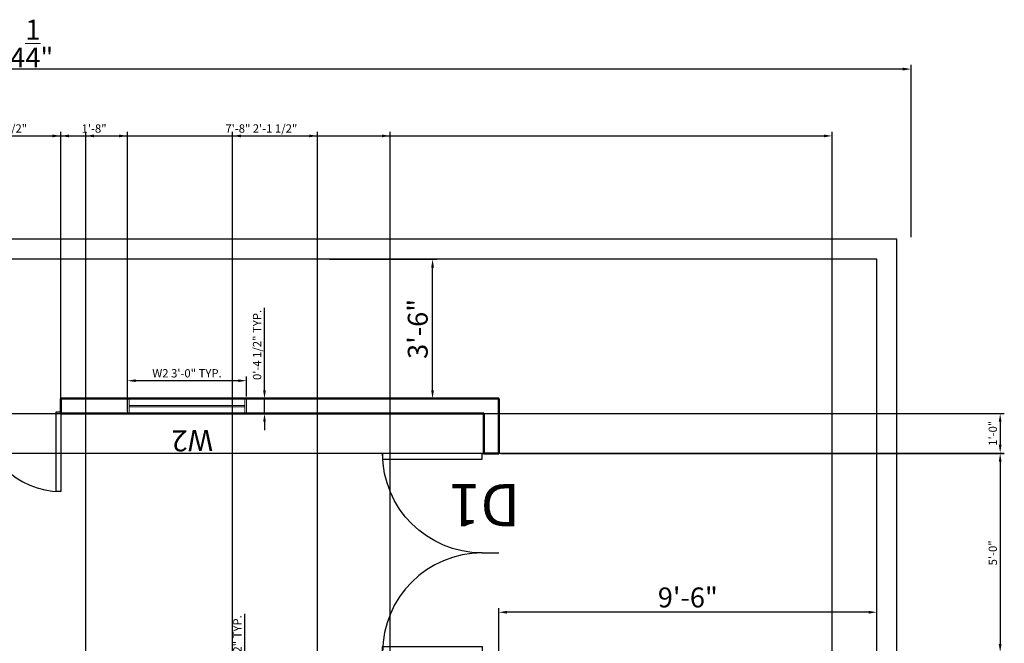
# Model space of a CAD drawing. Units: inches. Extents: x 1989 to 2637, y 1032 to 1611.
# Tile 5 of 5: x 2340 to 2637, y 1423 to 1611. Entities that reach past the tile are written whole.
import ezdxf

# ---------------------------------------------------------------- set-up
doc = ezdxf.new("R2010")
doc.units = ezdxf.units.IN
for name, color, linetype, lineweight in [('A-ANNO-TEXT', 1, 'Continuous', 18), ('C-PROP', 7, 'Continuous', 25), ('DIMENSIONS', 7, 'Continuous', 18), ('doors', 5, 'Continuous', 25), ('walls', 7, 'Continuous', 50), ('windows', 3, 'Continuous', 18)]:
    doc.layers.add(name, color=color, linetype=linetype, lineweight=lineweight)
doc.styles.get("Standard").update_dxf_attribs({"font": 'arial.ttf'})
doc.dimstyles.new('ISO-25', dxfattribs={"dimtxt": 2.5, "dimasz": 2.5, "dimexe": 1.25, "dimexo": 0.625, "dimtad": 1, "dimlunit": 4, "dimtxsty": 'Standard', "dimcen": 2.5, "dimadec": 0, "dimazin": 0, "dimtfac": 1, "dimtmove": 0, "dimatfit": 3, "dimfxl": 1, "dimarcsym": 0})

# ---------------------------------------------------------------- blocks, each defined once
blk = doc.blocks.new('*U2')
for p, q in [((0, 0), (0, -5)), ((30, 0), (30, -5))]:
    blk.add_line(p, q)
blk.add_lwpolyline([(0, 0), (0, 30), (1.75, 30), (1.75, 0)], close=True)
blk.add_arc((0, 0), 30, 0, 90)
blk = doc.blocks.new('*D12')
at = {"layer": 'Defpoints', "color": 0, "transparency": 16777216}
for p in [(2064.5, 1596.21), (2064.5, 1544.92), (2608.81, 1544.92)]:
    blk.add_point(p, dxfattribs=at)
at = {"layer": 'DIMENSIONS', "color": 0, "lineweight": -2, "transparency": 16777216}
for p, q in [((2064.5, 1545.55), (2064.5, 1597.46)), ((2608.81, 1545.55), (2608.81, 1597.46)), ((2606.31, 1596.21), (2067, 1596.21))]:
    blk.add_line(p, q, dxfattribs=at)
at = {"layer": 'DIMENSIONS', "color": 0, "transparency": 16777216}
for points in [[(2067, 1596.63), (2067, 1595.79), (2064.5, 1596.21)], [(2606.31, 1596.63), (2606.31, 1595.79), (2608.81, 1596.21)]]:
    blk.add_solid(points, dxfattribs=at)
at = {"layer": 'DIMENSIONS', "color": 0, "transparency": 16777216, "insert": (2336.65, 1603.9), "char_height": 6, "attachment_point": 5}
blk.add_mtext('45\'-4{\\H1x;\\S1/4;}"', dxfattribs=at)
blk = doc.blocks.new('*D13')
at = {"layer": 'Defpoints', "color": 0, "transparency": 16777216}
for p in [(2484.5, 1432.53), (2484.5, 1402.72), (2598.5, 1403.71)]:
    blk.add_point(p, dxfattribs=at)
at = {"layer": 'DIMENSIONS', "color": 0, "lineweight": -2, "transparency": 16777216}
for p, q in [((2484.5, 1403.34), (2484.5, 1433.78)), ((2598.5, 1404.33), (2598.5, 1433.78)), ((2596, 1432.53), (2487, 1432.53))]:
    blk.add_line(p, q, dxfattribs=at)
at = {"layer": 'DIMENSIONS', "color": 0, "transparency": 16777216}
for points in [[(2487, 1432.95), (2487, 1432.12), (2484.5, 1432.53)], [(2596, 1432.95), (2596, 1432.12), (2598.5, 1432.53)]]:
    blk.add_solid(points, dxfattribs=at)
at = {"layer": 'DIMENSIONS', "color": 0, "transparency": 16777216, "insert": (2541.5, 1436.22), "char_height": 6, "attachment_point": 5}
blk.add_mtext('9\'-6"', dxfattribs=at)
blk = doc.blocks.new('*D14')
at = {"layer": 'Defpoints', "color": 0, "transparency": 16777216}
for p in [(2432.92, 1538.92), (2464.56, 1538.92), (2432.92, 1496.92)]:
    blk.add_point(p, dxfattribs=at)
at = {"layer": 'DIMENSIONS', "color": 0, "lineweight": -2, "transparency": 16777216}
for p, q in [((2433.54, 1538.92), (2465.81, 1538.92)), ((2464.56, 1499.42), (2464.56, 1536.42)), ((2433.54, 1496.92), (2465.81, 1496.92))]:
    blk.add_line(p, q, dxfattribs=at)
at = {"layer": 'DIMENSIONS', "color": 0, "transparency": 16777216}
for points in [[(2464.14, 1536.42), (2464.98, 1536.42), (2464.56, 1538.92)], [(2464.14, 1499.42), (2464.98, 1499.42), (2464.56, 1496.92)]]:
    blk.add_solid(points, dxfattribs=at)
at = {"layer": 'DIMENSIONS', "color": 0, "transparency": 16777216, "insert": (2460.87, 1517.92), "char_height": 6, "attachment_point": 5, "rotation": 90}
blk.add_mtext('3\'-6"', dxfattribs=at)
blk = doc.blocks.new('WIN-W2-36IN')
for p, q in [((0, 0), (0, 35.95)), ((0, 35.95), (4.5, 35.95)), ((4.5, 35.95), (4.5, 0)), ((0, 35.45), (4.5, 35.45)), ((2.05, 35.45), (2.05, 0.5)), ((2.45, 35.45), (2.45, 0.5)), ((4.5, 0.5), (0, 0.5)), ((4.5, 0), (0, 0))]:
    blk.add_line(p, q)
blk = doc.blocks.new('*D26')
at = {"layer": 'Defpoints', "color": 0, "transparency": 16777216}
for p in [(2372.56, 1502.31), (2372.56, 1496.92), (2408.51, 1496.92)]:
    blk.add_point(p, dxfattribs=at)
at = {"layer": 'DIMENSIONS', "color": 0, "lineweight": -2, "transparency": 16777216}
for p, q in [((2372.56, 1497.55), (2372.56, 1503.56)), ((2406.01, 1502.31), (2375.06, 1502.31)), ((2408.51, 1497.55), (2408.51, 1503.56))]:
    blk.add_line(p, q, dxfattribs=at)
at = {"layer": 'DIMENSIONS', "color": 0, "transparency": 16777216}
for points in [[(2375.06, 1502.73), (2375.06, 1501.9), (2372.56, 1502.31)], [(2406.01, 1502.73), (2406.01, 1501.9), (2408.51, 1502.31)]]:
    blk.add_solid(points, dxfattribs=at)
at = {"layer": 'DIMENSIONS', "color": 0, "transparency": 16777216, "insert": (2390.54, 1504.22), "char_height": 2.5, "attachment_point": 5}
blk.add_mtext('W2 3\'-0" TYP.', dxfattribs=at)
blk = doc.blocks.new('*D27')
at = {"layer": 'Defpoints', "color": 0, "transparency": 16777216}
for p in [(2408.51, 1496.92), (2413.9, 1496.92), (2408.51, 1492.42)]:
    blk.add_point(p, dxfattribs=at)
at = {"layer": 'DIMENSIONS', "color": 0, "lineweight": -2, "transparency": 16777216}
for p, q in [((2413.9, 1499.42), (2413.9, 1524.23)), ((2409.14, 1496.92), (2415.15, 1496.92)), ((2413.9, 1492.42), (2413.9, 1496.92)), ((2409.14, 1492.42), (2415.15, 1492.42)), ((2413.9, 1489.92), (2413.9, 1487.42))]:
    blk.add_line(p, q, dxfattribs=at)
at = {"layer": 'DIMENSIONS', "color": 0, "transparency": 16777216}
for points in [[(2413.49, 1499.42), (2414.32, 1499.42), (2413.9, 1496.92)], [(2413.49, 1489.92), (2414.32, 1489.92), (2413.9, 1492.42)]]:
    blk.add_solid(points, dxfattribs=at)
at = {"layer": 'DIMENSIONS', "color": 0, "transparency": 16777216, "insert": (2411.99, 1513.08), "char_height": 2.5, "attachment_point": 5, "rotation": 90}
blk.add_mtext('0\'-4 1/2" TYP.', dxfattribs=at)
blk = doc.blocks.new('*D29')
at = {"layer": 'Defpoints', "color": 0, "transparency": 16777216}
for p in [(2407.97, 1407.51), (2411.12, 1407.51), (2411.12, 1390.17)]:
    blk.add_point(p, dxfattribs=at)
at = {"layer": 'DIMENSIONS', "color": 0, "lineweight": -2, "transparency": 16777216}
for p, q in [((2407.97, 1407.51), (2407.97, 1432.09)), ((2410.49, 1407.51), (2406.72, 1407.51)), ((2407.97, 1392.67), (2407.97, 1405.01)), ((2410.49, 1390.17), (2406.72, 1390.17))]:
    blk.add_line(p, q, dxfattribs=at)
at = {"layer": 'DIMENSIONS', "color": 0, "transparency": 16777216}
for points in [[(2407.55, 1405.01), (2408.39, 1405.01), (2407.97, 1407.51)], [(2407.55, 1392.67), (2408.39, 1392.67), (2407.97, 1390.17)]]:
    blk.add_solid(points, dxfattribs=at)
at = {"layer": 'DIMENSIONS', "color": 0, "transparency": 16777216, "insert": (2406.05, 1421.05), "char_height": 2.5, "attachment_point": 5, "rotation": 90}
blk.add_mtext('1\'-5 1/2" TYP.', dxfattribs=at)
blk = doc.blocks.new('*D40')
at = {"layer": 'Defpoints', "color": 0, "transparency": 16777216}
for p in [(2585, 1576.07), (2082.5, 1496.92), (2585, 1310.92)]:
    blk.add_point(p, dxfattribs=at)
at = {"layer": 'DIMENSIONS', "color": 0, "lineweight": -2, "transparency": 16777216}
for p, q in [((2082.5, 1497.55), (2082.5, 1577.32)), ((2085, 1576.07), (2582.5, 1576.07)), ((2585, 1311.55), (2585, 1577.32))]:
    blk.add_line(p, q, dxfattribs=at)
at = {"layer": 'DIMENSIONS', "color": 0, "transparency": 16777216}
for points in [[(2085, 1576.49), (2085, 1575.65), (2082.5, 1576.07)], [(2582.5, 1576.49), (2582.5, 1575.65), (2585, 1576.07)]]:
    blk.add_solid(points, dxfattribs=at)
at = {"layer": 'DIMENSIONS', "color": 0, "transparency": 16777216, "insert": (2333.75, 1577.99), "char_height": 2.5, "attachment_point": 5}
blk.add_mtext('41\'-10 1/2"', dxfattribs=at)
blk = doc.blocks.new('*D42')
at = {"layer": 'Defpoints', "color": 0, "transparency": 16777216}
for p in [(2484.5, 1480.42), (2484.5, 1420.42), (2635.65, 1420.42)]:
    blk.add_point(p, dxfattribs=at)
at = {"layer": 'DIMENSIONS', "color": 0, "lineweight": -2, "transparency": 16777216}
for p, q in [((2485.12, 1480.42), (2636.9, 1480.42)), ((2635.65, 1477.92), (2635.65, 1422.92)), ((2485.12, 1420.42), (2636.9, 1420.42))]:
    blk.add_line(p, q, dxfattribs=at)
at = {"layer": 'DIMENSIONS', "color": 0, "transparency": 16777216}
for points in [[(2635.23, 1477.92), (2636.06, 1477.92), (2635.65, 1480.42)], [(2635.23, 1422.92), (2636.06, 1422.92), (2635.65, 1420.42)]]:
    blk.add_solid(points, dxfattribs=at)
at = {"layer": 'DIMENSIONS', "color": 0, "transparency": 16777216, "insert": (2633.75, 1450.42), "char_height": 2.5, "attachment_point": 5, "rotation": 90}
blk.add_mtext('5\'-0"', dxfattribs=at)
blk = doc.blocks.new('*D44')
at = {"layer": 'Defpoints', "color": 0, "transparency": 16777216}
for p in [(2352.5, 1576.07), (2304.5, 1496.92), (2352.5, 1496.92)]:
    blk.add_point(p, dxfattribs=at)
at = {"layer": 'DIMENSIONS', "color": 0, "lineweight": -2, "transparency": 16777216}
for p, q in [((2304.5, 1497.55), (2304.5, 1577.32)), ((2307, 1576.07), (2350, 1576.07)), ((2352.5, 1497.55), (2352.5, 1577.32))]:
    blk.add_line(p, q, dxfattribs=at)
at = {"layer": 'DIMENSIONS', "color": 0, "transparency": 16777216}
for points in [[(2307, 1576.49), (2307, 1575.65), (2304.5, 1576.07)], [(2350, 1576.49), (2350, 1575.65), (2352.5, 1576.07)]]:
    blk.add_solid(points, dxfattribs=at)
at = {"layer": 'DIMENSIONS', "color": 0, "transparency": 16777216, "insert": (2328.5, 1577.97), "char_height": 2.5, "attachment_point": 5}
blk.add_mtext('4\'-0"', dxfattribs=at)
blk = doc.blocks.new('*D50')
at = {"layer": 'Defpoints', "color": 0, "transparency": 16777216}
for p in [(2087, 1492.42), (2087, 1480.5), (2635.65, 1480.5)]:
    blk.add_point(p, dxfattribs=at)
at = {"layer": 'DIMENSIONS', "color": 0, "lineweight": -2, "transparency": 16777216}
for p, q in [((2087.62, 1492.42), (2636.9, 1492.42)), ((2635.65, 1489.92), (2635.65, 1483)), ((2087.62, 1480.5), (2636.9, 1480.5))]:
    blk.add_line(p, q, dxfattribs=at)
at = {"layer": 'DIMENSIONS', "color": 0, "transparency": 16777216}
for points in [[(2635.23, 1489.92), (2636.06, 1489.92), (2635.65, 1492.42)], [(2635.23, 1483), (2636.06, 1483), (2635.65, 1480.5)]]:
    blk.add_solid(points, dxfattribs=at)
at = {"layer": 'DIMENSIONS', "color": 0, "transparency": 16777216, "insert": (2633.75, 1486.46), "char_height": 2.5, "attachment_point": 5, "rotation": 90}
blk.add_mtext('1\'-0"', dxfattribs=at)
blk = doc.blocks.new('*D54')
at = {"layer": 'Defpoints', "color": 0, "transparency": 16777216}
for p in [(2429.87, 1576.07), (2404.3, 1358.98), (2429.87, 1358.98)]:
    blk.add_point(p, dxfattribs=at)
at = {"layer": 'DIMENSIONS', "color": 0, "lineweight": -2, "transparency": 16777216}
for p, q in [((2404.3, 1359.6), (2404.3, 1577.32)), ((2406.8, 1576.07), (2427.37, 1576.07)), ((2429.87, 1359.6), (2429.87, 1577.32))]:
    blk.add_line(p, q, dxfattribs=at)
at = {"layer": 'DIMENSIONS', "color": 0, "transparency": 16777216}
for points in [[(2406.8, 1576.49), (2406.8, 1575.65), (2404.3, 1576.07)], [(2427.37, 1576.49), (2427.37, 1575.65), (2429.87, 1576.07)]]:
    blk.add_solid(points, dxfattribs=at)
at = {"layer": 'DIMENSIONS', "color": 0, "transparency": 16777216, "insert": (2417.08, 1577.99), "char_height": 2.5, "attachment_point": 5}
blk.add_mtext('2\'-1 1/2"', dxfattribs=at)
blk = doc.blocks.new('*D56')
at = {"layer": 'Defpoints', "color": 0, "transparency": 16777216}
for p in [(2372.56, 1576.07), (2352.5, 1492.42), (2372.56, 1492.42)]:
    blk.add_point(p, dxfattribs=at)
at = {"layer": 'DIMENSIONS', "color": 0, "lineweight": -2, "transparency": 16777216}
for p, q in [((2352.5, 1493.05), (2352.5, 1577.32)), ((2355, 1576.07), (2370.06, 1576.07)), ((2372.56, 1493.05), (2372.56, 1577.32))]:
    blk.add_line(p, q, dxfattribs=at)
at = {"layer": 'DIMENSIONS', "color": 0, "transparency": 16777216}
for points in [[(2355, 1576.49), (2355, 1575.65), (2352.5, 1576.07)], [(2370.06, 1576.49), (2370.06, 1575.65), (2372.56, 1576.07)]]:
    blk.add_solid(points, dxfattribs=at)
at = {"layer": 'DIMENSIONS', "color": 0, "transparency": 16777216, "insert": (2362.53, 1577.97), "char_height": 2.5, "attachment_point": 5}
blk.add_mtext('1\'-8"', dxfattribs=at)
blk = doc.blocks.new('*D60')
at = {"layer": 'Defpoints', "color": 0, "transparency": 16777216}
for p in [(2451.78, 1576.07), (2360, 1087.42), (2451.78, 1087.42)]:
    blk.add_point(p, dxfattribs=at)
at = {"layer": 'DIMENSIONS', "color": 0, "lineweight": -2, "transparency": 16777216}
for p, q in [((2360, 1088.05), (2360, 1577.32)), ((2362.5, 1576.07), (2449.28, 1576.07)), ((2451.78, 1088.05), (2451.78, 1577.32))]:
    blk.add_line(p, q, dxfattribs=at)
at = {"layer": 'DIMENSIONS', "color": 0, "transparency": 16777216}
for points in [[(2362.5, 1576.49), (2362.5, 1575.65), (2360, 1576.07)], [(2449.28, 1576.49), (2449.28, 1575.65), (2451.78, 1576.07)]]:
    blk.add_solid(points, dxfattribs=at)
at = {"layer": 'DIMENSIONS', "color": 0, "transparency": 16777216, "insert": (2405.89, 1577.97), "char_height": 2.5, "attachment_point": 5}
blk.add_mtext('7\'-8"', dxfattribs=at)

msp = doc.modelspace()

# ---------------------------------------------------------------- linework, layer by layer
at = {"layer": 'C-PROP'}
for p, q in [((2604.498, 1544.921), (2064.498, 1544.921)), ((2604.498, 1064.921), (2604.498, 1544.921)), ((2598.498, 1538.921), (2070.498, 1538.921)), ((2598.498, 1070.921), (2598.498, 1538.921))]:
    msp.add_line(p, q, dxfattribs=at)
at = {"layer": 'walls'}
for p, q in [((2352.498, 1492.421), (2352.498, 1496.921)), ((2352.498, 1496.921), (2484.498, 1496.921)), ((2484.498, 1496.921), (2484.498, 1480.421)), ((2352.498, 1492.421), (2479.998, 1492.421)), ((2479.998, 1492.421), (2479.998, 1480.421)), ((2479.998, 1480.421), (2484.498, 1480.421))]:
    msp.add_line(p, q, dxfattribs=at)

# ---------------------------------------------------------------- block references
at = {"layer": 'doors', "xscale": 0.8, "yscale": 0.8, "zscale": 0.8, "rotation": 180}
msp.add_blockref('*U2', (2352.498, 1492.921), dxfattribs=at)
at = {"layer": 'doors', "xscale": -1, "rotation": 90}
msp.add_blockref('*U2', (2479.498, 1480.421), dxfattribs=at)
at = {"layer": 'doors', "rotation": 89.99999999999999}
msp.add_blockref('*U2', (2479.498, 1420.421), dxfattribs=at)
at = {"layer": 'windows', "rotation": 89.99999999999706}
msp.add_blockref('WIN-W2-36IN', (2408.51, 1492.421), dxfattribs=at)

# ---------------------------------------------------------------- texts
at = {"layer": 'A-ANNO-TEXT', "attachment_point": 1}
for s, width, gutter_width, insert, char_height, rotation in [('W2', 5.29651, 31.753, (2398.397, 1481.128), 6.3507, 180.67334), ('D1', 3.801, 63.542, (2490.988, 1458.436), 12.7085, 180)]:
    msp.add_mtext_dynamic_manual_height_columns(s, width=width, gutter_width=gutter_width, heights=[0], dxfattribs=dict(at, insert=insert, char_height=char_height, rotation=rotation))

# ---------------------------------------------------------------- dimensions: what is measured, and where the dimension line sits
at = {"layer": 'DIMENSIONS'}
for base, p1, p2, override, picture, middle in [((2064.498, 1596.209), (2608.808, 1544.921), (2064.498, 1544.921), {"dimtxt": 6, "dimclrd": 0, "dimclre": 0, "dimclrt": 0}, '*D12', (2336.653, 1603.898)), ((2584.998, 1576.071), (2082.498, 1496.921), (2584.998, 1310.921), {"dimdec": 1, "dimlfac": 1, "dimrnd": 0, "dimzin": 1, "dimdsep": 46, "dimlunit": 4, "dimfrac": 2}, '*D40', (2333.748, 1577.989)), ((2352.498, 1576.071), (2304.498, 1496.921), (2352.498, 1496.921), {"dimdec": 1, "dimlfac": 1, "dimrnd": 0, "dimzin": 1, "dimdsep": 46, "dimlunit": 4, "dimfrac": 2}, '*D44', (2328.498, 1577.972)), ((2372.561, 1576.071), (2352.498, 1492.421), (2372.561, 1492.421), {"dimdec": 1, "dimlfac": 1, "dimrnd": 0, "dimzin": 1, "dimdsep": 46, "dimlunit": 4, "dimfrac": 2}, '*D56', (2362.529, 1577.972)), ((2451.776, 1576.071), (2359.998, 1087.421), (2451.776, 1087.421), {"dimdec": 1, "dimlfac": 1, "dimrnd": 0, "dimzin": 1, "dimdsep": 46, "dimlunit": 4, "dimfrac": 2}, '*D60', (2405.887, 1577.972)), ((2429.87, 1576.071), (2404.299, 1358.979), (2429.87, 1358.979), {"dimdec": 1, "dimlfac": 1, "dimrnd": 0, "dimzin": 1, "dimdsep": 46, "dimlunit": 4, "dimfrac": 2}, '*D54', (2417.084, 1577.989)), ((2484.498, 1432.534), (2598.498, 1403.705), (2484.498, 1402.719), {"dimtxt": 6, "dimclrd": 0, "dimclre": 0, "dimclrt": 0}, '*D13', (2541.498, 1436.223))]:
    dim = msp.add_linear_dim(base=base, p1=p1, p2=p2, dimstyle='ISO-25', override=override, dxfattribs=at)
    dim.commit()
    dim.dimension.update_dxf_attribs({"geometry": picture, "text_midpoint": middle})
for base, p1, p2, override, picture, middle in [((2464.559, 1538.921), (2432.917, 1496.921), (2432.917, 1538.921), {"dimtxt": 6, "dimclrd": 0, "dimclre": 0, "dimclrt": 0}, '*D14', (2460.869, 1517.921)), ((2635.648, 1480.504), (2086.998, 1492.421), (2086.998, 1480.504), {"dimdec": 1, "dimlfac": 1, "dimrnd": 0, "dimzin": 1, "dimdsep": 46, "dimlunit": 4, "dimfrac": 2}, '*D50', (2633.746, 1486.463)), ((2635.648, 1420.421), (2484.498, 1480.421), (2484.498, 1420.421), {"dimdec": 1, "dimlfac": 1, "dimrnd": 0, "dimzin": 1, "dimdsep": 46, "dimlunit": 4, "dimfrac": 2}, '*D42', (2633.746, 1450.421))]:
    dim = msp.add_linear_dim(base=base, p1=p1, p2=p2, angle=90, dimstyle='ISO-25', override=override, dxfattribs=at)
    dim.commit()
    dim.dimension.update_dxf_attribs({"geometry": picture, "text_midpoint": middle})
for base, p1, p2, angle, text, picture, middle in [((2413.903, 1496.921), (2408.51, 1492.421), (2408.51, 1496.921), 90, '<> TYP.', '*D27', (2411.985, 1513.078)), ((2372.561, 1502.313), (2408.51, 1496.921), (2372.561, 1496.921), 180, 'W2 <> TYP.', '*D26', (2390.536, 1504.216)), ((2407.969, 1407.508), (2411.119, 1390.175), (2411.119, 1407.508), 90, '<> TYP.', '*D29', (2406.051, 1421.047))]:
    dim = msp.add_linear_dim(base=base, p1=p1, p2=p2, angle=angle, text=text, dimstyle='ISO-25', override={"dimdec": 1, "dimlfac": 1, "dimrnd": 0, "dimzin": 1, "dimdsep": 46, "dimlunit": 4, "dimfrac": 2}, dxfattribs=at)
    dim.commit()
    dim.dimension.update_dxf_attribs({"geometry": picture, "text_midpoint": middle})

doc.saveas('drawing.dxf')
